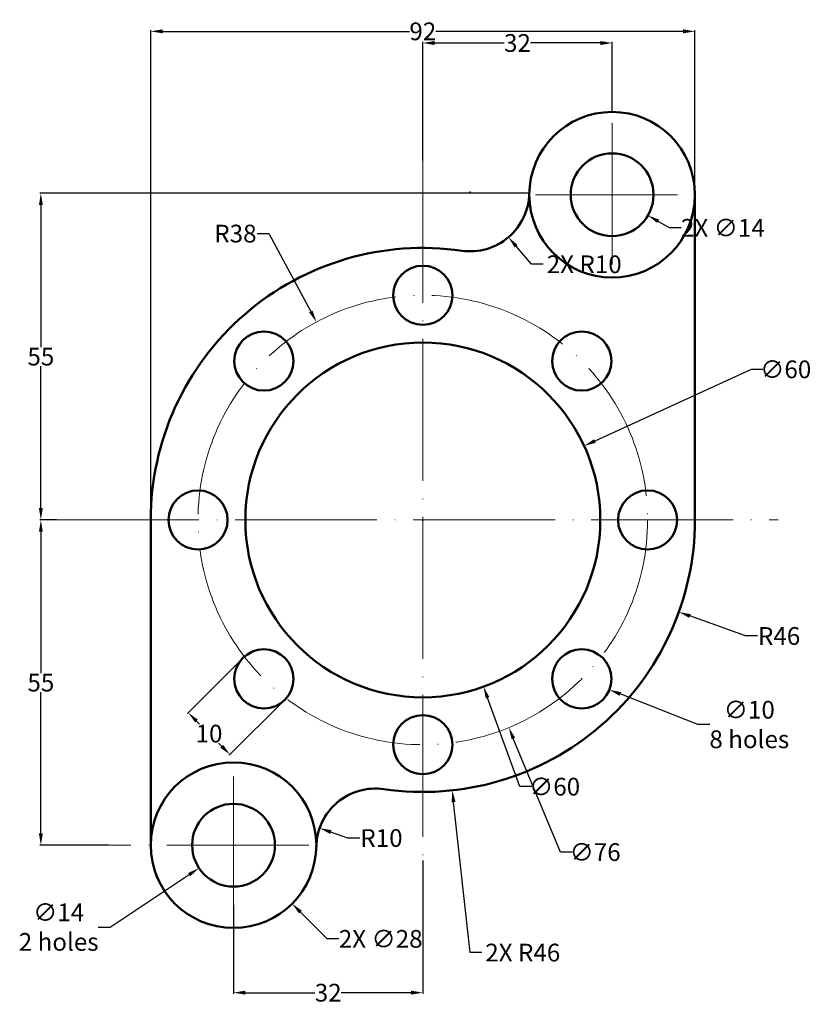
# Model space of a CAD drawing. Units: inches. Extents: x 127 to 261, y 46 to 213.
import ezdxf

# ---------------------------------------------------------------- set-up
doc = ezdxf.new("R2010")
doc.units = ezdxf.units.IN
doc.header["$MEASUREMENT"] = 0
doc.linetypes.add('ACAD_ISO04W100', pattern=[30, 24, -3, 0, -3])
for name, color, linetype, lineweight in [('M-CNTR', 4, 'ACAD_ISO04W100', 18), ('M-DIMS', 2, 'Continuous', 25), ('M-OUTL', 7, 'Continuous', 50)]:
    doc.layers.add(name, color=color, linetype=linetype, lineweight=lineweight)
doc.styles.get("Standard").update_dxf_attribs({"font": 'arial.ttf'})
doc.dimstyles.get("Standard").update_dxf_attribs({"dimtxt": 3, "dimasz": 2, "dimexe": 0.18, "dimexo": 0.0625, "dimgap": 0.09, "dimtad": 0, "dimtih": 1, "dimtoh": 1, "dimdec": 0, "dimzin": 0, "dimdsep": 46, "dimtxsty": 'Standard', "dimcen": 0.09, "dimclrd": 1, "dimclre": 1, "dimadec": 0, "dimazin": 0, "dimtfac": 1, "dimtdec": 0, "dimtofl": 0, "dimtmove": 0, "dimatfit": 3, "dimfxl": 1, "dimtolj": 1, "dimtzin": 0, "dimarcsym": 0})

# ---------------------------------------------------------------- blocks, each defined once
blk = doc.blocks.new('*D1')
at = {"layer": 'Defpoints', "color": 0, "transparency": 16777216}
for p in [(194.87, 70.38), (162.87, 62.93), (162.87, 47.99)]:
    blk.add_point(p, dxfattribs=at)
at = {"layer": 'M-DIMS', "color": 0, "lineweight": -2, "transparency": 16777216}
for p, q in [((194.87, 70.32), (194.87, 47.81)), ((162.87, 62.87), (162.87, 47.81)), ((164.87, 47.99), (176.64, 47.99)), ((192.87, 47.99), (181.09, 47.99))]:
    blk.add_line(p, q, dxfattribs=at)
at = {"layer": 'M-DIMS', "color": 0, "transparency": 16777216}
for points in [[(164.87, 48.33), (164.87, 47.66), (162.87, 47.99)], [(192.87, 48.33), (192.87, 47.66), (194.87, 47.99)]]:
    blk.add_solid(points, dxfattribs=at)
at = {"layer": 'M-DIMS', "color": 0, "transparency": 16777216, "insert": (178.87, 47.99), "char_height": 3, "attachment_point": 5}
blk.add_mtext('\\A1;32', dxfattribs=at)
blk = doc.blocks.new('*U2')
blk.add_circle((0, 0), 5)
blk = doc.blocks.new('*U3')
at = {"layer": 'M-OUTL', "color": 0, "linetype": 'ByBlock', "lineweight": -2, "transparency": 16777216}
for p, rotation in [((194.87, 165.93), 90), ((168, 154.8), 135), ((221.74, 154.8), 45), ((156.87, 127.93), 180), ((168, 101.06), 225), ((221.74, 101.06), 314.9999999999999), ((194.87, 89.93), 270)]:
    blk.add_blockref('*U2', p, dxfattribs=dict(at, rotation=rotation))
blk.add_blockref('*U2', (232.87, 127.93), dxfattribs=at)
blk = doc.blocks.new('*D4')
at = {"layer": 'Defpoints', "color": 0, "transparency": 16777216}
for p in [(177.43, 75.82), (186.86, 72.51)]:
    blk.add_point(p, dxfattribs=at)
at = {"layer": 'M-DIMS', "color": 0, "lineweight": -2, "transparency": 16777216}
for p, q in [((182.21, 74.14), (179.31, 75.16)), ((184.21, 74.14), (182.21, 74.14))]:
    blk.add_line(p, q, dxfattribs=at)
at = {"layer": 'M-DIMS', "color": 0, "transparency": 16777216}
blk.add_solid([(179.42, 75.47), (179.2, 74.84), (177.43, 75.82)], dxfattribs=at)
at = {"layer": 'M-DIMS', "color": 0, "transparency": 16777216, "insert": (187.88, 74.14), "char_height": 3, "attachment_point": 5}
blk.add_mtext('\\A1;R10', dxfattribs=at)
blk = doc.blocks.new('*D5')
at = {"layer": 'Defpoints', "color": 0, "transparency": 16777216}
for p in [(168.7, 76.81), (157.04, 69.06)]:
    blk.add_point(p, dxfattribs=at)
at = {"layer": 'M-DIMS', "color": 0, "lineweight": -2, "transparency": 16777216}
for p, q in [((162.78, 72.93), (162.96, 72.93)), ((162.87, 72.84), (162.87, 73.02)), ((142.01, 59.08), (155.37, 67.95)), ((140.01, 59.08), (142.01, 59.08))]:
    blk.add_line(p, q, dxfattribs=at)
at = {"layer": 'M-DIMS', "color": 0, "transparency": 16777216}
blk.add_solid([(155.19, 68.23), (155.55, 67.68), (157.04, 69.06)], dxfattribs=at)
at = {"layer": 'M-DIMS', "color": 0, "transparency": 16777216, "insert": (133.31, 59.08), "char_height": 3, "attachment_point": 5}
blk.add_mtext('\\A1;∅14\\P2 holes', dxfattribs=at)
blk = doc.blocks.new('*D6')
at = {"layer": 'Defpoints', "color": 0, "transparency": 16777216}
for p in [(226.87, 208.59), (226.87, 196.93), (194.87, 188.66)]:
    blk.add_point(p, dxfattribs=at)
at = {"layer": 'M-DIMS', "color": 0, "lineweight": -2, "transparency": 16777216}
for p, q in [((194.87, 188.72), (194.87, 208.77)), ((196.87, 208.59), (208.64, 208.59)), ((224.87, 208.59), (213.09, 208.59)), ((226.87, 197), (226.87, 208.77))]:
    blk.add_line(p, q, dxfattribs=at)
at = {"layer": 'M-DIMS', "color": 0, "transparency": 16777216}
for points in [[(196.87, 208.92), (196.87, 208.25), (194.87, 208.59)], [(224.87, 208.92), (224.87, 208.25), (226.87, 208.59)]]:
    blk.add_solid(points, dxfattribs=at)
at = {"layer": 'M-DIMS', "color": 0, "transparency": 16777216, "insert": (210.87, 208.59), "char_height": 3, "attachment_point": 5}
blk.add_mtext('\\A1;32', dxfattribs=at)
blk = doc.blocks.new('*D7')
at = {"layer": 'Defpoints', "color": 0, "transparency": 16777216}
for p in [(212.87, 183.18), (130.3, 127.93), (133.02, 127.93)]:
    blk.add_point(p, dxfattribs=at)
at = {"layer": 'M-DIMS', "color": 0, "lineweight": -2, "transparency": 16777216}
for p, q in [((212.81, 183.18), (130.12, 183.18)), ((130.3, 181.18), (130.3, 157.17)), ((130.3, 129.93), (130.3, 153.94)), ((132.96, 127.93), (130.12, 127.93))]:
    blk.add_line(p, q, dxfattribs=at)
at = {"layer": 'M-DIMS', "color": 0, "transparency": 16777216}
for points in [[(129.97, 181.18), (130.63, 181.18), (130.3, 183.18)], [(129.97, 129.93), (130.63, 129.93), (130.3, 127.93)]]:
    blk.add_solid(points, dxfattribs=at)
at = {"layer": 'M-DIMS', "color": 0, "transparency": 16777216, "insert": (130.3, 155.56), "char_height": 3, "attachment_point": 5}
blk.add_mtext('\\A1;55', dxfattribs=at)
blk = doc.blocks.new('*D8')
at = {"layer": 'Defpoints', "color": 0, "transparency": 16777216}
for p in [(130.3, 127.93), (133.02, 127.93), (142, 72.93)]:
    blk.add_point(p, dxfattribs=at)
at = {"layer": 'M-DIMS', "color": 0, "lineweight": -2, "transparency": 16777216}
for p, q in [((132.96, 127.93), (130.12, 127.93)), ((130.3, 125.93), (130.3, 102.05)), ((130.3, 74.93), (130.3, 98.82)), ((141.93, 72.93), (130.12, 72.93))]:
    blk.add_line(p, q, dxfattribs=at)
at = {"layer": 'M-DIMS', "color": 0, "transparency": 16777216}
for points in [[(129.97, 125.93), (130.63, 125.93), (130.3, 127.93)], [(129.97, 74.93), (130.63, 74.93), (130.3, 72.93)]]:
    blk.add_solid(points, dxfattribs=at)
at = {"layer": 'M-DIMS', "color": 0, "transparency": 16777216, "insert": (130.3, 100.43), "char_height": 3, "attachment_point": 5}
blk.add_mtext('\\A1;55', dxfattribs=at)
blk = doc.blocks.new('*D9')
at = {"layer": 'Defpoints', "color": 0, "transparency": 16777216}
for p in [(222.13, 140.45), (167.6, 115.42)]:
    blk.add_point(p, dxfattribs=at)
at = {"layer": 'M-DIMS', "color": 0, "lineweight": -2, "transparency": 16777216}
for p, q in [((250.36, 153.4), (223.95, 141.28)), ((252.36, 153.4), (250.36, 153.4)), ((194.78, 127.93), (194.96, 127.93)), ((194.87, 127.84), (194.87, 128.02))]:
    blk.add_line(p, q, dxfattribs=at)
at = {"layer": 'M-DIMS', "color": 0, "transparency": 16777216}
blk.add_solid([(223.81, 141.59), (224.09, 140.98), (222.13, 140.45)], dxfattribs=at)
at = {"layer": 'M-DIMS', "color": 0, "transparency": 16777216, "insert": (256.22, 153.4), "char_height": 3, "attachment_point": 5}
blk.add_mtext('\\A1;∅60', dxfattribs=at)
blk = doc.blocks.new('*D10')
at = {"layer": 'Defpoints', "color": 0, "transparency": 16777216}
for p in [(194.87, 127.93), (238.15, 112.36)]:
    blk.add_point(p, dxfattribs=at)
at = {"layer": 'M-DIMS', "color": 0, "lineweight": -2, "transparency": 16777216}
for p, q in [((194.78, 127.93), (194.96, 127.93)), ((194.87, 127.84), (194.87, 128.02)), ((249.42, 108.31), (240.03, 111.69)), ((251.42, 108.31), (249.42, 108.31))]:
    blk.add_line(p, q, dxfattribs=at)
at = {"layer": 'M-DIMS', "color": 0, "transparency": 16777216}
blk.add_solid([(240.15, 112), (239.92, 111.37), (238.15, 112.36)], dxfattribs=at)
at = {"layer": 'M-DIMS', "color": 0, "transparency": 16777216, "insert": (255.1, 108.31), "char_height": 3, "attachment_point": 5}
blk.add_mtext('\\A1;R46', dxfattribs=at)
blk = doc.blocks.new('*D11')
at = {"layer": 'Defpoints', "color": 0, "transparency": 16777216}
for p in [(217.08, 102.89), (226.39, 99.23)]:
    blk.add_point(p, dxfattribs=at)
at = {"layer": 'M-DIMS', "color": 0, "lineweight": -2, "transparency": 16777216}
for p, q in [((221.65, 101.06), (221.83, 101.06)), ((221.74, 100.97), (221.74, 101.15)), ((241.38, 93.34), (228.25, 98.5)), ((243.38, 93.34), (241.38, 93.34))]:
    blk.add_line(p, q, dxfattribs=at)
at = {"layer": 'M-DIMS', "color": 0, "transparency": 16777216}
blk.add_solid([(228.37, 98.81), (228.13, 98.19), (226.39, 99.23)], dxfattribs=at)
at = {"layer": 'M-DIMS', "color": 0, "transparency": 16777216, "insert": (250.06, 93.34), "char_height": 3, "attachment_point": 5}
blk.add_mtext('\\A1;∅10\\P8 holes', dxfattribs=at)
blk = doc.blocks.new('*D12')
at = {"layer": 'Defpoints', "color": 0, "transparency": 16777216}
for p in [(176.89, 161.41), (194.87, 127.93)]:
    blk.add_point(p, dxfattribs=at)
at = {"layer": 'M-DIMS', "color": 0, "lineweight": -2, "transparency": 16777216}
for p, q in [((166.86, 176.36), (168.86, 176.36)), ((168.86, 176.36), (175.95, 163.18)), ((194.78, 127.93), (194.96, 127.93)), ((194.87, 127.84), (194.87, 128.02))]:
    blk.add_line(p, q, dxfattribs=at)
at = {"layer": 'M-DIMS', "color": 0, "transparency": 16777216}
blk.add_solid([(176.24, 163.33), (175.65, 163.02), (176.89, 161.41)], dxfattribs=at)
at = {"layer": 'M-DIMS', "color": 0, "transparency": 16777216, "insert": (163.19, 176.36), "char_height": 3, "attachment_point": 5}
blk.add_mtext('\\A1;R38', dxfattribs=at)
blk = doc.blocks.new('MOUNTING-LUG')
for radius in [14, 7]:
    blk.add_circle((14, 14), radius)
blk = doc.blocks.new('*D14')
at = {"layer": 'Defpoints', "color": 0, "transparency": 16777216}
for p in [(240.87, 210.56), (240.87, 182.93), (148.87, 127.93)]:
    blk.add_point(p, dxfattribs=at)
at = {"layer": 'M-DIMS', "color": 1, "lineweight": -2, "transparency": 16777216}
for p, q in [((148.87, 128), (148.87, 210.74)), ((150.87, 210.56), (192.64, 210.56)), ((238.87, 210.56), (197.09, 210.56)), ((240.87, 183), (240.87, 210.74))]:
    blk.add_line(p, q, dxfattribs=at)
at = {"layer": 'M-DIMS', "color": 1, "transparency": 16777216}
for points in [[(150.87, 210.9), (150.87, 210.23), (148.87, 210.56)], [(238.87, 210.9), (238.87, 210.23), (240.87, 210.56)]]:
    blk.add_solid(points, dxfattribs=at)
at = {"layer": 'M-DIMS', "color": 0, "transparency": 16777216, "insert": (194.87, 210.56), "char_height": 3, "attachment_point": 5}
blk.add_mtext('\\A1;92', dxfattribs=at)
blk = doc.blocks.new('*D15')
at = {"layer": 'Defpoints', "color": 0, "transparency": 16777216}
for p in [(164.46, 104.6), (171.53, 97.53), (155.2, 95.34)]:
    blk.add_point(p, dxfattribs=at)
at = {"layer": 'M-DIMS', "color": 1, "lineweight": -2, "transparency": 16777216}
for p, q in [((164.42, 104.56), (155.07, 95.21)), ((171.49, 97.48), (162.14, 88.14)), ((156.61, 93.92), (157.11, 93.42)), ((160.85, 89.68), (160.35, 90.18))]:
    blk.add_line(p, q, dxfattribs=at)
at = {"layer": 'M-DIMS', "color": 1, "transparency": 16777216}
for points in [[(156.85, 94.16), (156.38, 93.69), (155.2, 95.34)], [(161.09, 89.92), (160.62, 89.44), (162.27, 88.27)]]:
    blk.add_solid(points, dxfattribs=at)
at = {"layer": 'M-DIMS', "color": 0, "transparency": 16777216, "insert": (158.73, 91.8), "char_height": 3, "attachment_point": 5}
blk.add_mtext('\\A1;10', dxfattribs=at)
blk = doc.blocks.new('*D16')
at = {"layer": 'Defpoints', "color": 0, "transparency": 16777216}
for p in [(152.97, 82.83), (172.77, 63.03)]:
    blk.add_point(p, dxfattribs=at)
at = {"layer": 'M-DIMS', "color": 1, "lineweight": -2, "transparency": 16777216}
for p, q in [((162.78, 72.93), (162.96, 72.93)), ((162.87, 72.84), (162.87, 73.02)), ((178.7, 57.09), (174.18, 61.62)), ((180.7, 57.09), (178.7, 57.09))]:
    blk.add_line(p, q, dxfattribs=at)
at = {"layer": 'M-DIMS', "color": 1, "transparency": 16777216}
blk.add_solid([(174.42, 61.86), (173.94, 61.38), (172.77, 63.03)], dxfattribs=at)
at = {"layer": 'M-DIMS', "color": 0, "transparency": 16777216, "insert": (187.75, 57.09), "char_height": 3, "attachment_point": 5}
blk.add_mtext('\\A1;2X ∅28', dxfattribs=at)
blk = doc.blocks.new('*D17')
at = {"layer": 'Defpoints', "color": 0, "transparency": 16777216}
for p in [(220.8, 186.43), (232.93, 179.43)]:
    blk.add_point(p, dxfattribs=at)
at = {"layer": 'M-DIMS', "color": 1, "lineweight": -2, "transparency": 16777216}
for p, q in [((226.78, 182.93), (226.96, 182.93)), ((226.87, 182.84), (226.87, 183.02)), ((236.57, 177.33), (234.66, 178.43)), ((238.57, 177.33), (236.57, 177.33))]:
    blk.add_line(p, q, dxfattribs=at)
at = {"layer": 'M-DIMS', "color": 1, "transparency": 16777216}
blk.add_solid([(234.83, 178.72), (234.49, 178.15), (232.93, 179.43)], dxfattribs=at)
at = {"layer": 'M-DIMS', "color": 0, "transparency": 16777216, "insert": (245.6, 177.33), "char_height": 3, "attachment_point": 5}
blk.add_mtext('\\A1;2X ∅14', dxfattribs=at)
blk = doc.blocks.new('*D18')
at = {"layer": 'Defpoints', "color": 0, "transparency": 16777216}
for p in [(202.87, 183.36), (209.35, 175.74)]:
    blk.add_point(p, dxfattribs=at)
at = {"layer": 'M-DIMS', "color": 1, "lineweight": -2, "transparency": 16777216}
for p, q in [((202.78, 183.36), (202.96, 183.36)), ((202.87, 183.27), (202.87, 183.45)), ((213.24, 171.17), (210.64, 174.22)), ((215.24, 171.17), (213.24, 171.17))]:
    blk.add_line(p, q, dxfattribs=at)
at = {"layer": 'M-DIMS', "color": 1, "transparency": 16777216}
blk.add_solid([(210.9, 174.43), (210.39, 174), (209.35, 175.74)], dxfattribs=at)
at = {"layer": 'M-DIMS', "color": 0, "transparency": 16777216, "insert": (222.15, 171.17), "char_height": 3, "attachment_point": 5}
blk.add_mtext('\\A1;2X R10', dxfattribs=at)
blk = doc.blocks.new('*D19')
at = {"layer": 'Defpoints', "color": 0, "transparency": 16777216}
for p in [(194.87, 127.93), (199.86, 82.21)]:
    blk.add_point(p, dxfattribs=at)
at = {"layer": 'M-DIMS', "color": 1, "lineweight": -2, "transparency": 16777216}
for p, q in [((194.78, 127.93), (194.96, 127.93)), ((194.87, 127.84), (194.87, 128.02)), ((202.85, 54.77), (200.07, 80.22)), ((204.85, 54.77), (202.85, 54.77))]:
    blk.add_line(p, q, dxfattribs=at)
at = {"layer": 'M-DIMS', "color": 1, "transparency": 16777216}
blk.add_solid([(200.4, 80.25), (199.74, 80.18), (199.86, 82.21)], dxfattribs=at)
at = {"layer": 'M-DIMS', "color": 0, "transparency": 16777216, "insert": (211.77, 54.77), "char_height": 3, "attachment_point": 5}
blk.add_mtext('\\A1;2X R46', dxfattribs=at)
blk = doc.blocks.new('*D20')
at = {"layer": 'Defpoints', "color": 0, "transparency": 16777216}
for p in [(184.61, 156.13), (205.13, 99.74)]:
    blk.add_point(p, dxfattribs=at)
at = {"layer": 'M-DIMS', "color": 1, "lineweight": -2, "transparency": 16777216}
for p, q in [((194.78, 127.93), (194.96, 127.93)), ((194.87, 127.84), (194.87, 128.02)), ((211.28, 82.83), (205.81, 97.86)), ((213.28, 82.83), (211.28, 82.83))]:
    blk.add_line(p, q, dxfattribs=at)
at = {"layer": 'M-DIMS', "color": 1, "transparency": 16777216}
blk.add_solid([(206.12, 97.98), (205.5, 97.75), (205.13, 99.74)], dxfattribs=at)
at = {"layer": 'M-DIMS', "color": 0, "transparency": 16777216, "insert": (217.15, 82.83), "char_height": 3, "attachment_point": 5}
blk.add_mtext('\\A1;∅60', dxfattribs=at)
blk = doc.blocks.new('*D21')
at = {"layer": 'Defpoints', "color": 0, "transparency": 16777216}
for p in [(180.32, 163.04), (209.41, 92.83)]:
    blk.add_point(p, dxfattribs=at)
at = {"layer": 'M-DIMS', "color": 1, "lineweight": -2, "transparency": 16777216}
for p, q in [((194.78, 127.93), (194.96, 127.93)), ((194.87, 127.84), (194.87, 128.02)), ((218.13, 71.76), (210.17, 90.98)), ((220.13, 71.76), (218.13, 71.76))]:
    blk.add_line(p, q, dxfattribs=at)
at = {"layer": 'M-DIMS', "color": 1, "transparency": 16777216}
blk.add_solid([(210.48, 91.11), (209.87, 90.85), (209.41, 92.83)], dxfattribs=at)
at = {"layer": 'M-DIMS', "color": 0, "transparency": 16777216, "insert": (224, 71.76), "char_height": 3, "attachment_point": 5}
blk.add_mtext('\\A1;∅76', dxfattribs=at)

msp = doc.modelspace()

# ---------------------------------------------------------------- linework, layer by layer
at = {"layer": 'M-CNTR'}
for p, q in [((226.87, 171.11), (226.87, 197.46)), ((194.87, 188.66), (194.87, 70.38)), ((213.93, 182.93), (240.87, 182.93)), ((133.02, 127.93), (254.94, 127.93)), ((162.87, 84.52), (162.87, 61.29)), ((175.59, 72.93), (142, 72.93))]:
    msp.add_line(p, q, dxfattribs=at)
msp.add_circle((194.87, 127.93), 38, dxfattribs=at)
at = {"layer": 'M-OUTL'}
for p, q in [((240.87, 127.93), (240.87, 182.93)), ((148.87, 127.93), (148.87, 72.93))]:
    msp.add_line(p, q, dxfattribs=at)
msp.add_circle((194.87, 127.93), 30, dxfattribs=at)
for centre, radius, start, end in [((202.87, 183.36), 10, 261.7829, 358.9851), ((194.87, 127.93), 46, 81.7829, 180), ((194.87, 127.93), 46, 261.7829, 0), ((186.86, 72.51), 10, 81.7829, 178.9851)]:
    msp.add_arc(centre, radius, start, end, dxfattribs=at)

# ---------------------------------------------------------------- block references
for name, p in [('MOUNTING-LUG', (212.87, 168.93)), ('*U3', (0, 0)), ('MOUNTING-LUG', (148.87, 58.93))]:
    msp.add_blockref(name, p, dxfattribs=at)

# ---------------------------------------------------------------- dimensions: what is measured, and where the dimension line sits
at = {"layer": 'M-DIMS'}
for base, p1, p2, override, picture, middle in [((240.87, 210.56), (148.87, 127.93), (240.87, 182.93), {"dimdec": 0, "dimlfac": 1, "dimrnd": 0, "dimzin": 0, "dimdsep": 46, "dimlunit": 2}, '*D14', (194.87, 210.56)), ((226.87, 208.59), (194.87, 188.66), (226.87, 196.93), {"dimclrd": 0, "dimclre": 0, "dimclrt": 0}, '*D6', (210.87, 208.59))]:
    dim = msp.add_linear_dim(base=base, p1=p1, p2=p2, dimstyle='Standard', override=override, dxfattribs=at)
    dim.commit()
    dim.dimension.update_dxf_attribs({"geometry": picture, "text_midpoint": middle})
for p1, p2, text, override, picture, middle in [((220.8, 186.43), (232.93, 179.43), '2X <>', {"dimdec": 0, "dimlfac": 1, "dimrnd": 0, "dimzin": 0, "dimdsep": 46, "dimlunit": 2}, '*D17', (245.6, 177.33)), ((217.08, 102.89), (226.39, 99.23), '<>\\P8 holes', {"dimclrd": 0, "dimclre": 0, "dimclrt": 0}, '*D11', (250.06, 93.34)), ((152.97, 82.83), (172.77, 63.03), '2X <>', {"dimdec": 0, "dimlfac": 1, "dimrnd": 0, "dimzin": 0, "dimdsep": 46, "dimlunit": 2}, '*D16', (187.75, 57.09)), ((168.7, 76.81), (157.04, 69.06), '<>\\P2 holes', {"dimclrd": 0, "dimclre": 0, "dimclrt": 0}, '*D5', (133.31, 59.08))]:
    dim = msp.add_diameter_dim_2p(p1=p1, p2=p2, text=text, dimstyle='Standard', override=override, dxfattribs=at)
    dim.commit()
    dim.dimension.update_dxf_attribs({"geometry": picture, "text_midpoint": middle, "dimtype": 163})
for base, p1, p2, angle, override, picture, middle in [((130.3, 127.93), (212.87, 183.18), (133.02, 127.93), 90, {"dimclrd": 0, "dimclre": 0, "dimclrt": 0}, '*D7', (130.3, 155.56)), ((130.3, 127.93), (142, 72.93), (133.02, 127.93), 90, {"dimclrd": 0, "dimclre": 0, "dimclrt": 0}, '*D8', (130.3, 100.43)), ((155.2, 95.34), (171.53, 97.53), (164.46, 104.6), 135, {"dimdec": 0, "dimlfac": 1, "dimrnd": 0, "dimzin": 0, "dimdsep": 46, "dimlunit": 2}, '*D15', (158.73, 91.8))]:
    dim = msp.add_linear_dim(base=base, p1=p1, p2=p2, angle=angle, dimstyle='Standard', override=override, dxfattribs=at)
    dim.commit()
    dim.dimension.update_dxf_attribs({"geometry": picture, "text_midpoint": middle})
for center, mpoint, picture, middle in [((202.87, 183.36), (209.35, 175.74), '*D18', (222.15, 171.17)), ((194.87, 127.93), (199.86, 82.21), '*D19', (211.77, 54.77))]:
    dim = msp.add_radius_dim(center=center, mpoint=mpoint, text='2X <>', dimstyle='Standard', override={"dimdec": 0, "dimlfac": 1, "dimrnd": 0, "dimzin": 0, "dimdsep": 46, "dimlunit": 2}, dxfattribs=at)
    dim.commit()
    dim.dimension.update_dxf_attribs({"geometry": picture, "text_midpoint": middle, "dimtype": 164})
for center, mpoint, picture, middle in [((194.87, 127.93), (176.89, 161.41), '*D12', (163.19, 176.36)), ((194.87, 127.93), (238.15, 112.36), '*D10', (255.1, 108.31)), ((186.86, 72.51), (177.43, 75.82), '*D4', (187.88, 74.14))]:
    dim = msp.add_radius_dim(center=center, mpoint=mpoint, dimstyle='Standard', override={"dimclrd": 0, "dimclre": 0, "dimclrt": 0}, dxfattribs=at)
    dim.commit()
    dim.dimension.update_dxf_attribs({"geometry": picture, "text_midpoint": middle, "dimtype": 164})
for p1, p2, override, picture, middle in [((180.32, 163.04), (209.41, 92.83), {"dimdec": 0, "dimlfac": 1, "dimrnd": 0, "dimzin": 0, "dimdsep": 46, "dimlunit": 2}, '*D21', (224, 71.76)), ((167.6, 115.42), (222.13, 140.45), {"dimclrd": 0, "dimclre": 0, "dimclrt": 0}, '*D9', (256.22, 153.4)), ((184.61, 156.13), (205.13, 99.74), {"dimdec": 0, "dimlfac": 1, "dimrnd": 0, "dimzin": 0, "dimdsep": 46, "dimlunit": 2}, '*D20', (217.15, 82.83))]:
    dim = msp.add_diameter_dim_2p(p1=p1, p2=p2, dimstyle='Standard', override=override, dxfattribs=at)
    dim.commit()
    dim.dimension.update_dxf_attribs({"geometry": picture, "text_midpoint": middle, "dimtype": 163})
dim = msp.add_linear_dim(base=(162.87, 47.99), p1=(194.87, 70.38), p2=(162.87, 62.93), dimstyle='Standard', override={"dimclrd": 0, "dimclre": 0, "dimclrt": 0}, dxfattribs=at)
dim.commit()
dim.dimension.update_dxf_attribs({"geometry": '*D1', "text_midpoint": (178.87, 47.99), "dimtype": 160})

doc.saveas('drawing.dxf')
